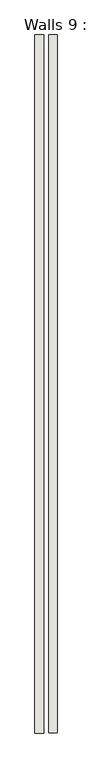
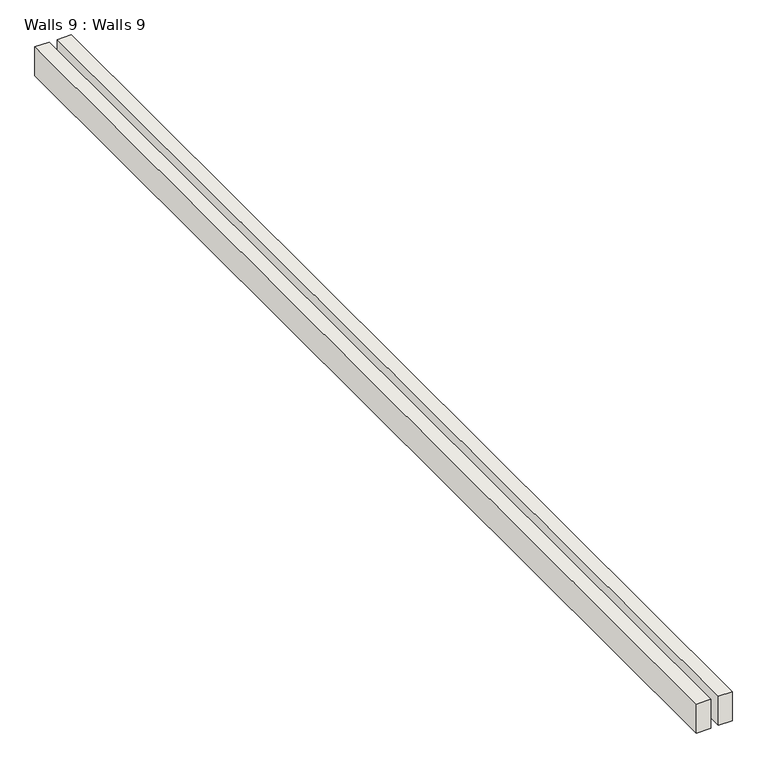
"""IFC4 building model written with IfcOpenShell, lengths in millimetres: wall geometry, Walls 9 : Walls 9."""

from ifc_helpers import new_model, si_unit, frame, origin, place, context, project, spatial, polyline, outline, extrude, source, transform, mapped, element, save


def walls_9_walls_9_70f34cfa(model_context):
    return source(origin(), model_context, "Body", "SweptSolid", [
        extrude(outline(polyline([(-12338.7432708, 11835.2893426), (-12338.7432708, 401.1257411), (-12482.0424966, 401.1257411), (-12482.0424966, 11835.2893426), (-12338.7432708, 11835.2893426)])), frame((0.0, 0.0, 3086.7795043), z_axis=(0.0, 0.0, 1.0), x_axis=(1.0, 0.0, 0.0)), (0.0, 0.0, 1.0), 304.8),
        extrude(outline(polyline([(-12118.8440117, 11835.2893426), (-12118.8440117, 409.864344), (-12258.517466, 409.864344), (-12258.517466, 11835.2893426), (-12118.8440117, 11835.2893426)])), frame((0.0, 0.0, 3086.7795043), z_axis=(0.0, 0.0, 1.0), x_axis=(1.0, 0.0, 0.0)), (0.0, 0.0, 1.0), 304.8),
    ])


if __name__ == "__main__":
    model = new_model("IFC4")
    model_context = context("Model", 3, world=origin())
    ifc_project = project(units=[si_unit("LENGTHUNIT", "METRE", prefix="MILLI")], contexts=[model_context])
    site = spatial("IfcSite", under=ifc_project)
    building = spatial("IfcBuilding", under=site)
    placement = place(None, origin())
    walls_9_walls_9_shape = walls_9_walls_9_70f34cfa(model_context)
    element("IfcWall", 1, ObjectType="Walls 9 : Walls 9", at=placement, inside=building, context=model_context, shape_type="MappedRepresentation", body=[
        mapped(walls_9_walls_9_shape, transform((0.0, 0.0, 0.0), x_axis=(1.0, 0.0, 0.0), y_axis=(0.0, 1.0, 0.0), z_axis=(0.0, 0.0, 1.0))),
    ])
    save(model, "model.ifc")

# Revit data of these elements
# Element 1 (IfcWall, "Walls 9 : Walls 9")
#   Materials on its faces: "Default Wall"
# Materials
#   "Default Wall": colour RGB 128 128 128, transparency 0
